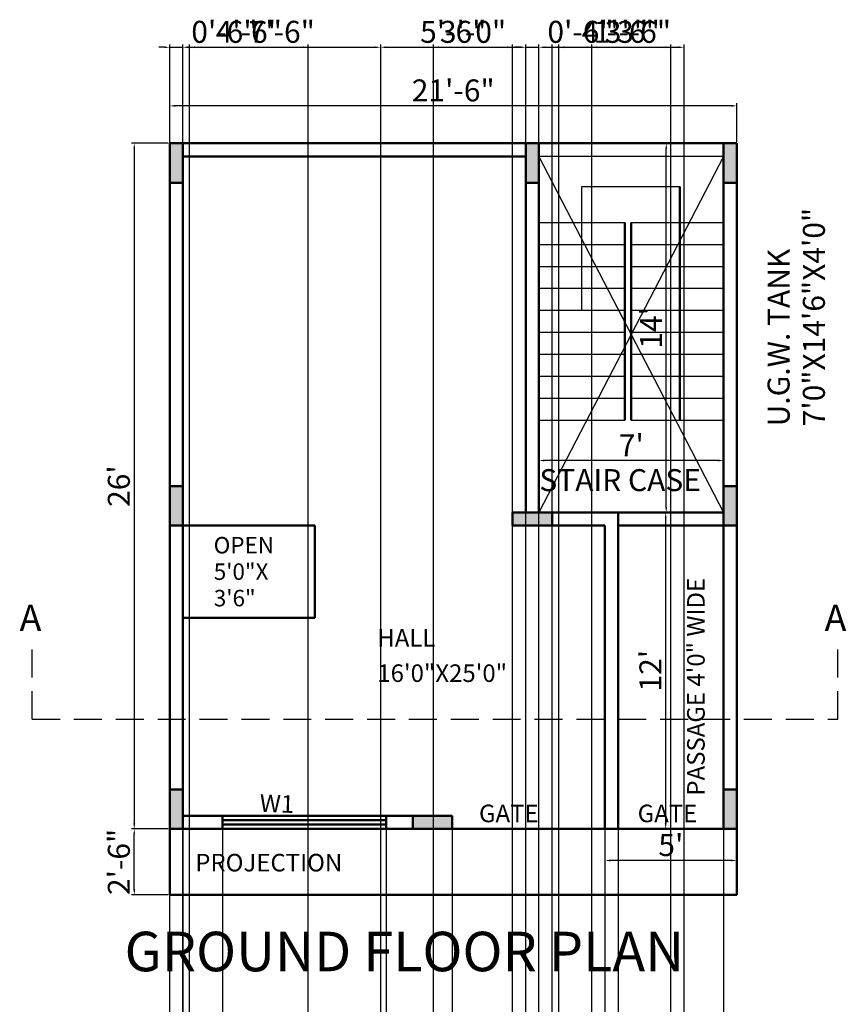
# Model space of a CAD drawing. Units: inches. Extents: x 2368 to 3882, y 1243 to 2139.
# Tile 3 of 6: x 2418 to 2794, y 1691 to 2139. Entities that reach past the tile are written whole.
import ezdxf

# ---------------------------------------------------------------- set-up
doc = ezdxf.new("R2010")
doc.units = ezdxf.units.IN
doc.linetypes.add('DASHED', pattern=[19.05, 12.7, -6.35])
for name, color, linetype, lineweight in [('A-ANNO-DIMS', 2, 'Continuous', 18), ('A-ANNO-SYMB', 1, 'DASHED', 25), ('A-ANNO-TEXT', 7, 'Continuous', 18), ('A-AREA-IDEN', 3, 'Continuous', 18), ('A-FLOR-STRS', 3, 'Continuous', 25), ('A-WALL', 7, 'Continuous', 50), ('A-WALL-PATT', 8, 'Continuous', 13)]:
    doc.layers.add(name, color=color, linetype=linetype, lineweight=lineweight)
doc.styles.get("Standard").update_dxf_attribs({"font": 'arial.ttf'})
doc.dimstyles.new('ISO-25', dxfattribs={"dimtxt": 10, "dimasz": 2.5, "dimexe": 1.25, "dimexo": 0.625, "dimtad": 1, "dimlunit": 3, "dimtxsty": 'Standard', "dimcen": 2.5, "dimadec": 0, "dimazin": 0, "dimtfac": 1, "dimtmove": 0, "dimatfit": 3, "dimfxl": 1, "dimarcsym": 0})

# ---------------------------------------------------------------- blocks, each defined once
blk = doc.blocks.new('*D1')
at = {"layer": 'A-ANNO-DIMS', "color": 0, "lineweight": -2, "transparency": 16777216}
for p, q in [((2486.5, 2083.43), (2486.5, 2101.09)), ((2742, 2099.84), (2489, 2099.84)), ((2744.5, 2083.43), (2744.5, 2101.09))]:
    blk.add_line(p, q, dxfattribs=at)
at = {"layer": 'A-ANNO-DIMS', "color": 0, "transparency": 16777216}
for points in [[(2489, 2100.26), (2489, 2099.43), (2486.5, 2099.84)], [(2742, 2100.26), (2742, 2099.43), (2744.5, 2099.84)]]:
    blk.add_solid(points, dxfattribs=at)
at = {"layer": 'Defpoints', "color": 0, "transparency": 16777216}
for p in [(2486.5, 2099.84), (2486.5, 2082.81), (2744.5, 2082.81)]:
    blk.add_point(p, dxfattribs=at)
at = {"layer": 'A-ANNO-DIMS', "color": 0, "transparency": 16777216, "insert": (2615.5, 2105.57), "char_height": 10, "attachment_point": 5}
blk.add_mtext('21\'-6"', dxfattribs=at)
blk = doc.blocks.new('*D2')
at = {"layer": 'A-ANNO-DIMS', "color": 0, "lineweight": -2, "transparency": 16777216}
for p, q in [((2654.5, 2076.18), (2654.5, 1937.22)), ((2738.5, 2076.18), (2738.5, 1937.22)), ((2736, 1938.47), (2657, 1938.47))]:
    blk.add_line(p, q, dxfattribs=at)
at = {"layer": 'A-ANNO-DIMS', "color": 0, "transparency": 16777216}
for points in [[(2657, 1938.88), (2657, 1938.05), (2654.5, 1938.47)], [(2736, 1938.88), (2736, 1938.05), (2738.5, 1938.47)]]:
    blk.add_solid(points, dxfattribs=at)
at = {"layer": 'Defpoints', "color": 0, "transparency": 16777216}
for p in [(2654.5, 2076.81), (2738.5, 2076.81), (2654.5, 1938.47)]:
    blk.add_point(p, dxfattribs=at)
at = {"layer": 'A-ANNO-DIMS', "color": 0, "transparency": 16777216, "insert": (2696.5, 1944.09), "char_height": 10, "attachment_point": 5}
blk.add_mtext("7'", dxfattribs=at)
blk = doc.blocks.new('*D3')
at = {"layer": 'A-ANNO-DIMS', "color": 0, "lineweight": -2, "transparency": 16777216}
for p, q in [((2649.12, 2082.81), (2713.65, 2082.81)), ((2712.4, 1917.31), (2712.4, 2080.31)), ((2649.12, 1914.81), (2713.65, 1914.81))]:
    blk.add_line(p, q, dxfattribs=at)
at = {"layer": 'A-ANNO-DIMS', "color": 0, "transparency": 16777216}
for points in [[(2711.99, 2080.31), (2712.82, 2080.31), (2712.4, 2082.81)], [(2711.99, 1917.31), (2712.82, 1917.31), (2712.4, 1914.81)]]:
    blk.add_solid(points, dxfattribs=at)
at = {"layer": 'Defpoints', "color": 0, "transparency": 16777216}
for p in [(2648.5, 2082.81), (2712.4, 2082.81), (2648.5, 1914.81)]:
    blk.add_point(p, dxfattribs=at)
at = {"layer": 'A-ANNO-DIMS', "color": 0, "transparency": 16777216, "insert": (2706.76, 1998.81), "char_height": 10, "attachment_point": 5, "rotation": 90}
blk.add_mtext("14'", dxfattribs=at)
blk = doc.blocks.new('*D4')
at = {"layer": 'A-ANNO-DIMS', "color": 0, "lineweight": -2, "transparency": 16777216}
for p, q in [((2485.87, 2082.81), (2469.15, 2082.81)), ((2470.4, 2080.31), (2470.4, 1773.31)), ((2485.87, 1770.81), (2469.15, 1770.81))]:
    blk.add_line(p, q, dxfattribs=at)
at = {"layer": 'A-ANNO-DIMS', "color": 0, "transparency": 16777216}
for points in [[(2469.98, 2080.31), (2470.82, 2080.31), (2470.4, 2082.81)], [(2469.98, 1773.31), (2470.82, 1773.31), (2470.4, 1770.81)]]:
    blk.add_solid(points, dxfattribs=at)
at = {"layer": 'Defpoints', "color": 0, "transparency": 16777216}
for p in [(2486.5, 2082.81), (2470.4, 1770.81), (2486.5, 1770.81)]:
    blk.add_point(p, dxfattribs=at)
at = {"layer": 'A-ANNO-DIMS', "color": 0, "transparency": 16777216, "insert": (2464.67, 1926.81), "char_height": 10, "attachment_point": 5, "rotation": 90}
blk.add_mtext("26'", dxfattribs=at)
blk = doc.blocks.new('*D5')
at = {"layer": 'A-ANNO-DIMS', "color": 0, "lineweight": -2, "transparency": 16777216}
for p, q in [((2485.87, 1770.81), (2469.15, 1770.81)), ((2470.4, 1743.31), (2470.4, 1768.31)), ((2485.87, 1740.81), (2469.15, 1740.81))]:
    blk.add_line(p, q, dxfattribs=at)
at = {"layer": 'A-ANNO-DIMS', "color": 0, "transparency": 16777216}
for points in [[(2469.98, 1768.31), (2470.82, 1768.31), (2470.4, 1770.81)], [(2469.98, 1743.31), (2470.82, 1743.31), (2470.4, 1740.81)]]:
    blk.add_solid(points, dxfattribs=at)
at = {"layer": 'Defpoints', "color": 0, "transparency": 16777216}
for p in [(2470.4, 1770.81), (2486.5, 1770.81), (2486.5, 1740.81)]:
    blk.add_point(p, dxfattribs=at)
at = {"layer": 'A-ANNO-DIMS', "color": 0, "transparency": 16777216, "insert": (2464.67, 1755.81), "char_height": 10, "attachment_point": 5, "rotation": 90}
blk.add_mtext('2\'-6"', dxfattribs=at)
blk = doc.blocks.new('*D6')
at = {"layer": 'A-ANNO-DIMS', "color": 0, "lineweight": -2, "transparency": 16777216}
for p, q in [((2684.5, 1770.18), (2684.5, 1755.19)), ((2744.5, 1770.18), (2744.5, 1755.19)), ((2742, 1756.44), (2687, 1756.44))]:
    blk.add_line(p, q, dxfattribs=at)
at = {"layer": 'A-ANNO-DIMS', "color": 0, "transparency": 16777216}
for points in [[(2687, 1756.85), (2687, 1756.02), (2684.5, 1756.44)], [(2742, 1756.85), (2742, 1756.02), (2744.5, 1756.44)]]:
    blk.add_solid(points, dxfattribs=at)
at = {"layer": 'Defpoints', "color": 0, "transparency": 16777216}
for p in [(2684.5, 1770.81), (2744.5, 1770.81), (2684.5, 1756.44)]:
    blk.add_point(p, dxfattribs=at)
at = {"layer": 'A-ANNO-DIMS', "color": 0, "transparency": 16777216, "insert": (2714.5, 1762.15), "char_height": 10, "attachment_point": 5}
blk.add_mtext("5'", dxfattribs=at)
blk = doc.blocks.new('*D7')
at = {"layer": 'A-ANNO-DIMS', "color": 0, "lineweight": -2, "transparency": 16777216}
for p, q in [((2691.12, 1914.81), (2713.39, 1914.81)), ((2712.14, 1773.31), (2712.14, 1912.31)), ((2691.12, 1770.81), (2713.39, 1770.81))]:
    blk.add_line(p, q, dxfattribs=at)
at = {"layer": 'A-ANNO-DIMS', "color": 0, "transparency": 16777216}
for points in [[(2711.72, 1912.31), (2712.55, 1912.31), (2712.14, 1914.81)], [(2711.72, 1773.31), (2712.55, 1773.31), (2712.14, 1770.81)]]:
    blk.add_solid(points, dxfattribs=at)
at = {"layer": 'Defpoints', "color": 0, "transparency": 16777216}
for p in [(2690.5, 1914.81), (2712.14, 1914.81), (2690.5, 1770.81)]:
    blk.add_point(p, dxfattribs=at)
at = {"layer": 'A-ANNO-DIMS', "color": 0, "transparency": 16777216, "insert": (2706.49, 1842.81), "char_height": 10, "attachment_point": 5, "rotation": 90}
blk.add_mtext("12'", dxfattribs=at)
blk = doc.blocks.new('*D32')
at = {"layer": 'A-ANNO-DIMS', "color": 0, "lineweight": -2, "transparency": 16777216}
for p, q in [((2484, 2126.51), (2481.5, 2126.51)), ((2486.5, 1909.43), (2486.5, 2127.76)), ((2486.5, 2126.51), (2492.5, 2126.51)), ((2492.5, 1909.43), (2492.5, 2127.76)), ((2495, 2126.51), (2525.33, 2126.51))]:
    blk.add_line(p, q, dxfattribs=at)
at = {"layer": 'A-ANNO-DIMS', "color": 0, "transparency": 16777216}
for points in [[(2484, 2126.93), (2484, 2126.09), (2486.5, 2126.51)], [(2495, 2126.93), (2495, 2126.09), (2492.5, 2126.51)]]:
    blk.add_solid(points, dxfattribs=at)
at = {"layer": 'Defpoints', "color": 0, "transparency": 16777216}
for p in [(2492.5, 2126.51), (2486.5, 1908.81), (2492.5, 1908.81)]:
    blk.add_point(p, dxfattribs=at)
at = {"layer": 'A-ANNO-DIMS', "color": 0, "transparency": 16777216, "insert": (2511.41, 2132.24), "char_height": 10, "attachment_point": 5}
blk.add_mtext('0\'-6"', dxfattribs=at)
blk = doc.blocks.new('*D33')
at = {"layer": 'A-ANNO-DIMS', "color": 0, "lineweight": -2, "transparency": 16777216}
for p, q in [((2510.5, 1776.18), (2510.5, 1251.93)), ((2492.5, 1770.18), (2492.5, 1251.93)), ((2495, 1253.18), (2508, 1253.18)), ((2510.5, 1253.18), (2539.89, 1253.18))]:
    blk.add_line(p, q, dxfattribs=at)
at = {"layer": 'A-ANNO-DIMS', "color": 0, "transparency": 16777216}
for points in [[(2495, 1253.6), (2495, 1252.77), (2492.5, 1253.18)], [(2508, 1253.6), (2508, 1252.77), (2510.5, 1253.18)]]:
    blk.add_solid(points, dxfattribs=at)
at = {"layer": 'Defpoints', "color": 0, "transparency": 16777216}
for p in [(2510.5, 1776.81), (2492.5, 1770.81), (2510.5, 1253.18)]:
    blk.add_point(p, dxfattribs=at)
at = {"layer": 'A-ANNO-DIMS', "color": 0, "transparency": 16777216, "insert": (2526.44, 1258.91), "char_height": 10, "attachment_point": 5}
blk.add_mtext('1\'-6"', dxfattribs=at)
blk = doc.blocks.new('*D34')
at = {"layer": 'A-ANNO-DIMS', "color": 0, "lineweight": -2, "transparency": 16777216}
for p, q in [((2510.5, 1776.18), (2510.5, 1251.93)), ((2585.04, 1776.18), (2585.04, 1251.93)), ((2513, 1253.18), (2582.54, 1253.18))]:
    blk.add_line(p, q, dxfattribs=at)
at = {"layer": 'A-ANNO-DIMS', "color": 0, "transparency": 16777216}
for points in [[(2513, 1253.6), (2513, 1252.77), (2510.5, 1253.18)], [(2582.54, 1253.6), (2582.54, 1252.77), (2585.04, 1253.18)]]:
    blk.add_solid(points, dxfattribs=at)
at = {"layer": 'Defpoints', "color": 0, "transparency": 16777216}
for p in [(2510.5, 1776.81), (2585.04, 1776.81), (2585.04, 1253.18)]:
    blk.add_point(p, dxfattribs=at)
at = {"layer": 'A-ANNO-DIMS', "color": 0, "transparency": 16777216, "insert": (2547.77, 1258.98), "char_height": 10, "attachment_point": 5}
blk.add_mtext('6\'-2 1/2"', dxfattribs=at)
blk = doc.blocks.new('*D35')
at = {"layer": 'A-ANNO-DIMS', "color": 0, "lineweight": -2, "transparency": 16777216}
for p, q in [((2585.04, 1776.18), (2585.04, 1251.93)), ((2615.04, 1776.18), (2615.04, 1251.93)), ((2587.54, 1253.18), (2612.54, 1253.18))]:
    blk.add_line(p, q, dxfattribs=at)
at = {"layer": 'A-ANNO-DIMS', "color": 0, "transparency": 16777216}
for points in [[(2587.54, 1253.6), (2587.54, 1252.77), (2585.04, 1253.18)], [(2612.54, 1253.6), (2612.54, 1252.77), (2615.04, 1253.18)]]:
    blk.add_solid(points, dxfattribs=at)
at = {"layer": 'Defpoints', "color": 0, "transparency": 16777216}
for p in [(2585.04, 1776.81), (2615.04, 1776.81), (2615.04, 1253.18)]:
    blk.add_point(p, dxfattribs=at)
at = {"layer": 'A-ANNO-DIMS', "color": 0, "transparency": 16777216, "insert": (2600.04, 1258.91), "char_height": 10, "attachment_point": 5}
blk.add_mtext('2\'-6"', dxfattribs=at)
blk = doc.blocks.new('*D36')
at = {"layer": 'A-ANNO-DIMS', "color": 0, "lineweight": -2, "transparency": 16777216}
for p, q in [((2615.04, 1776.18), (2615.04, 1251.93)), ((2684.5, 1770.18), (2684.5, 1251.93)), ((2617.54, 1253.18), (2682, 1253.18))]:
    blk.add_line(p, q, dxfattribs=at)
at = {"layer": 'A-ANNO-DIMS', "color": 0, "transparency": 16777216}
for points in [[(2617.54, 1253.6), (2617.54, 1252.77), (2615.04, 1253.18)], [(2682, 1253.6), (2682, 1252.77), (2684.5, 1253.18)]]:
    blk.add_solid(points, dxfattribs=at)
at = {"layer": 'Defpoints', "color": 0, "transparency": 16777216}
for p in [(2615.04, 1776.81), (2684.5, 1770.81), (2684.5, 1253.18)]:
    blk.add_point(p, dxfattribs=at)
at = {"layer": 'A-ANNO-DIMS', "color": 0, "transparency": 16777216, "insert": (2649.77, 1258.98), "char_height": 10, "attachment_point": 5}
blk.add_mtext('5\'-9 1/2"', dxfattribs=at)
blk = doc.blocks.new('*D37')
at = {"layer": 'A-ANNO-DIMS', "color": 0, "lineweight": -2, "transparency": 16777216}
for p, q in [((2690.5, 1770.18), (2690.5, 1251.93)), ((2738.5, 1770.18), (2738.5, 1251.93)), ((2693, 1253.18), (2736, 1253.18))]:
    blk.add_line(p, q, dxfattribs=at)
at = {"layer": 'A-ANNO-DIMS', "color": 0, "transparency": 16777216}
for points in [[(2693, 1253.6), (2693, 1252.77), (2690.5, 1253.18)], [(2736, 1253.6), (2736, 1252.77), (2738.5, 1253.18)]]:
    blk.add_solid(points, dxfattribs=at)
at = {"layer": 'Defpoints', "color": 0, "transparency": 16777216}
for p in [(2690.5, 1770.81), (2738.5, 1770.81), (2738.5, 1253.18)]:
    blk.add_point(p, dxfattribs=at)
at = {"layer": 'A-ANNO-DIMS', "color": 0, "transparency": 16777216, "insert": (2714.5, 1258.91), "char_height": 10, "attachment_point": 5}
blk.add_mtext('4\'-0"', dxfattribs=at)
blk = doc.blocks.new('*D39')
at = {"layer": 'A-ANNO-DIMS', "color": 0, "lineweight": -2, "transparency": 16777216}
for p, q in [((2484, 2126.51), (2481.5, 2126.51)), ((2486.5, 1639.51), (2486.5, 2127.76)), ((2486.5, 2126.51), (2492.5, 2126.51)), ((2492.5, 1633.51), (2492.5, 2127.76)), ((2495, 2126.51), (2525.33, 2126.51))]:
    blk.add_line(p, q, dxfattribs=at)
at = {"layer": 'A-ANNO-DIMS', "color": 0, "transparency": 16777216}
for points in [[(2484, 2126.93), (2484, 2126.09), (2486.5, 2126.51)], [(2495, 2126.93), (2495, 2126.09), (2492.5, 2126.51)]]:
    blk.add_solid(points, dxfattribs=at)
at = {"layer": 'Defpoints', "color": 0, "transparency": 16777216}
for p in [(2492.5, 2126.51), (2486.5, 1638.88), (2492.5, 1632.88)]:
    blk.add_point(p, dxfattribs=at)
at = {"layer": 'A-ANNO-DIMS', "color": 0, "transparency": 16777216, "insert": (2511.41, 2132.24), "char_height": 10, "attachment_point": 5}
blk.add_mtext('0\'-6"', dxfattribs=at)
blk = doc.blocks.new('*D50')
at = {"layer": 'A-ANNO-DIMS', "color": 0, "lineweight": -2, "transparency": 16777216}
for p, q in [((2582.5, 1633.51), (2582.5, 2127.76)), ((2585, 2126.51), (2646, 2126.51)), ((2648.5, 1639.51), (2648.5, 2127.76))]:
    blk.add_line(p, q, dxfattribs=at)
at = {"layer": 'A-ANNO-DIMS', "color": 0, "transparency": 16777216}
for points in [[(2585, 2126.93), (2585, 2126.09), (2582.5, 2126.51)], [(2646, 2126.93), (2646, 2126.09), (2648.5, 2126.51)]]:
    blk.add_solid(points, dxfattribs=at)
at = {"layer": 'Defpoints', "color": 0, "transparency": 16777216}
for p in [(2648.5, 2126.51), (2648.5, 1638.88), (2582.5, 1632.88)]:
    blk.add_point(p, dxfattribs=at)
at = {"layer": 'A-ANNO-DIMS', "color": 0, "transparency": 16777216, "insert": (2615.5, 2132.24), "char_height": 10, "attachment_point": 5}
blk.add_mtext('5\'-6"', dxfattribs=at)
blk = doc.blocks.new('*D51')
at = {"layer": 'A-ANNO-DIMS', "color": 0, "lineweight": -2, "transparency": 16777216}
for p, q in [((2646, 2126.51), (2643.5, 2126.51)), ((2648.5, 1639.51), (2648.5, 2127.76)), ((2648.5, 2126.51), (2654.5, 2126.51)), ((2654.5, 1639.51), (2654.5, 2127.76)), ((2657, 2126.51), (2687.33, 2126.51))]:
    blk.add_line(p, q, dxfattribs=at)
at = {"layer": 'A-ANNO-DIMS', "color": 0, "transparency": 16777216}
for points in [[(2646, 2126.93), (2646, 2126.09), (2648.5, 2126.51)], [(2657, 2126.93), (2657, 2126.09), (2654.5, 2126.51)]]:
    blk.add_solid(points, dxfattribs=at)
at = {"layer": 'Defpoints', "color": 0, "transparency": 16777216}
for p in [(2654.5, 2126.51), (2648.5, 1638.88), (2654.5, 1638.88)]:
    blk.add_point(p, dxfattribs=at)
at = {"layer": 'A-ANNO-DIMS', "color": 0, "transparency": 16777216, "insert": (2673.41, 2132.24), "char_height": 10, "attachment_point": 5}
blk.add_mtext('0\'-6"', dxfattribs=at)
blk = doc.blocks.new('*D52')
at = {"layer": 'A-ANNO-DIMS', "color": 0, "lineweight": -2, "transparency": 16777216}
for p, q in [((2492.5, 1633.51), (2492.5, 2127.76)), ((2495, 2126.51), (2580, 2126.51)), ((2582.5, 1633.51), (2582.5, 2127.76))]:
    blk.add_line(p, q, dxfattribs=at)
at = {"layer": 'A-ANNO-DIMS', "color": 0, "transparency": 16777216}
for points in [[(2495, 2126.93), (2495, 2126.09), (2492.5, 2126.51)], [(2580, 2126.93), (2580, 2126.09), (2582.5, 2126.51)]]:
    blk.add_solid(points, dxfattribs=at)
at = {"layer": 'Defpoints', "color": 0, "transparency": 16777216}
for p in [(2582.5, 2126.51), (2492.5, 1632.88), (2582.5, 1632.88)]:
    blk.add_point(p, dxfattribs=at)
at = {"layer": 'A-ANNO-DIMS', "color": 0, "transparency": 16777216, "insert": (2537.5, 2132.24), "char_height": 10, "attachment_point": 5}
blk.add_mtext('7\'-6"', dxfattribs=at)
blk = doc.blocks.new('*D53')
at = {"layer": 'A-ANNO-DIMS', "color": 0, "lineweight": -2, "transparency": 16777216}
for p, q in [((2663.5, 1357.51), (2663.5, 2127.76)), ((2666, 2126.51), (2712, 2126.51)), ((2714.5, 1357.51), (2714.5, 2127.76))]:
    blk.add_line(p, q, dxfattribs=at)
at = {"layer": 'A-ANNO-DIMS', "color": 0, "transparency": 16777216}
for points in [[(2666, 2126.93), (2666, 2126.09), (2663.5, 2126.51)], [(2712, 2126.93), (2712, 2126.09), (2714.5, 2126.51)]]:
    blk.add_solid(points, dxfattribs=at)
at = {"layer": 'Defpoints', "color": 0, "transparency": 16777216}
for p in [(2714.5, 2126.51), (2663.5, 1356.88), (2714.5, 1356.88)]:
    blk.add_point(p, dxfattribs=at)
at = {"layer": 'A-ANNO-DIMS', "color": 0, "transparency": 16777216, "insert": (2689, 2132.24), "char_height": 10, "attachment_point": 5}
blk.add_mtext('4\'-3"', dxfattribs=at)
blk = doc.blocks.new('*D58')
at = {"layer": 'A-ANNO-DIMS', "color": 0, "lineweight": -2, "transparency": 16777216}
for p, q in [((2495.5, 1471.51), (2495.5, 2127.76)), ((2498, 2126.51), (2547, 2126.51)), ((2549.5, 1471.51), (2549.5, 2127.76))]:
    blk.add_line(p, q, dxfattribs=at)
at = {"layer": 'A-ANNO-DIMS', "color": 0, "transparency": 16777216}
for points in [[(2498, 2126.93), (2498, 2126.09), (2495.5, 2126.51)], [(2547, 2126.93), (2547, 2126.09), (2549.5, 2126.51)]]:
    blk.add_solid(points, dxfattribs=at)
at = {"layer": 'Defpoints', "color": 0, "transparency": 16777216}
for p in [(2549.5, 2126.51), (2495.5, 1470.88), (2549.5, 1470.88)]:
    blk.add_point(p, dxfattribs=at)
at = {"layer": 'A-ANNO-DIMS', "color": 0, "transparency": 16777216, "insert": (2522.5, 2132.24), "char_height": 10, "attachment_point": 5}
blk.add_mtext('4\'-6"', dxfattribs=at)
blk = doc.blocks.new('*D59')
at = {"layer": 'A-ANNO-DIMS', "color": 0, "lineweight": -2, "transparency": 16777216}
for p, q in [((2606.5, 1465.51), (2606.5, 2127.76)), ((2609, 2126.51), (2640, 2126.51)), ((2642.5, 1471.51), (2642.5, 2127.76))]:
    blk.add_line(p, q, dxfattribs=at)
at = {"layer": 'A-ANNO-DIMS', "color": 0, "transparency": 16777216}
for points in [[(2609, 2126.93), (2609, 2126.09), (2606.5, 2126.51)], [(2640, 2126.93), (2640, 2126.09), (2642.5, 2126.51)]]:
    blk.add_solid(points, dxfattribs=at)
at = {"layer": 'Defpoints', "color": 0, "transparency": 16777216}
for p in [(2642.5, 2126.51), (2642.5, 1470.88), (2606.5, 1464.88)]:
    blk.add_point(p, dxfattribs=at)
at = {"layer": 'A-ANNO-DIMS', "color": 0, "transparency": 16777216, "insert": (2624.5, 2132.24), "char_height": 10, "attachment_point": 5}
blk.add_mtext('3\'-0"', dxfattribs=at)
blk = doc.blocks.new('*D60')
at = {"layer": 'A-ANNO-DIMS', "color": 0, "lineweight": -2, "transparency": 16777216}
for p, q in [((2660.5, 1471.51), (2660.5, 2127.76)), ((2663, 2126.51), (2676, 2126.51)), ((2678.5, 1471.51), (2678.5, 2127.76)), ((2678.5, 2126.51), (2707.89, 2126.51))]:
    blk.add_line(p, q, dxfattribs=at)
at = {"layer": 'A-ANNO-DIMS', "color": 0, "transparency": 16777216}
for points in [[(2663, 2126.93), (2663, 2126.09), (2660.5, 2126.51)], [(2676, 2126.93), (2676, 2126.09), (2678.5, 2126.51)]]:
    blk.add_solid(points, dxfattribs=at)
at = {"layer": 'Defpoints', "color": 0, "transparency": 16777216}
for p in [(2678.5, 2126.51), (2660.5, 1470.88), (2678.5, 1470.88)]:
    blk.add_point(p, dxfattribs=at)
at = {"layer": 'A-ANNO-DIMS', "color": 0, "transparency": 16777216, "insert": (2694.44, 2132.24), "char_height": 10, "attachment_point": 5}
blk.add_mtext('1\'-6"', dxfattribs=at)
blk = doc.blocks.new('*D61')
at = {"layer": 'A-ANNO-DIMS', "color": 0, "lineweight": -2, "transparency": 16777216}
for p, q in [((2678.5, 1471.51), (2678.5, 2127.76)), ((2681, 2126.51), (2718, 2126.51)), ((2720.5, 1471.51), (2720.5, 2127.76))]:
    blk.add_line(p, q, dxfattribs=at)
at = {"layer": 'A-ANNO-DIMS', "color": 0, "transparency": 16777216}
for points in [[(2681, 2126.93), (2681, 2126.09), (2678.5, 2126.51)], [(2718, 2126.93), (2718, 2126.09), (2720.5, 2126.51)]]:
    blk.add_solid(points, dxfattribs=at)
at = {"layer": 'Defpoints', "color": 0, "transparency": 16777216}
for p in [(2720.5, 2126.51), (2678.5, 1470.88), (2720.5, 1470.88)]:
    blk.add_point(p, dxfattribs=at)
at = {"layer": 'A-ANNO-DIMS', "color": 0, "transparency": 16777216, "insert": (2699.5, 2132.24), "char_height": 10, "attachment_point": 5}
blk.add_mtext('3\'-6"', dxfattribs=at)

msp = doc.modelspace()

# ---------------------------------------------------------------- hatches: boundary and pattern name
at = {"layer": 'A-WALL-PATT'}
h = msp.add_hatch(color=256, dxfattribs=at)
h.dxf.hatch_style = 1
h.paths.add_polyline_path([(2492.497, 1344.883), (2486.497, 1344.883), (2486.497, 1326.883), (2492.497, 1326.883)])
h.paths.add_polyline_path([(2618.497, 1332.883), (2600.497, 1332.883), (2600.497, 1326.883), (2618.497, 1326.883)])
h.paths.add_polyline_path([(2744.497, 1344.883), (2738.497, 1344.883), (2738.497, 1326.883), (2744.497, 1326.883)])
h.paths.add_polyline_path([(2744.497, 1482.883), (2738.497, 1482.883), (2738.497, 1464.883), (2744.497, 1464.883)])
h.paths.add_polyline_path([(2660.497, 1470.883), (2642.497, 1470.883), (2642.497, 1464.883), (2660.497, 1464.883)])
h.paths.add_polyline_path([(2492.497, 1482.883), (2486.497, 1482.883), (2486.497, 1464.883), (2492.497, 1464.883)])
h.paths.add_polyline_path([(2492.497, 1638.883), (2486.497, 1638.883), (2486.497, 1620.883), (2492.497, 1620.883)])
h.paths.add_polyline_path([(2654.497, 1638.883), (2648.497, 1638.883), (2648.497, 1620.883), (2654.497, 1620.883)])
h.paths.add_polyline_path([(2744.497, 1638.883), (2738.497, 1638.883), (2738.497, 1620.883), (2744.497, 1620.883)])
h.paths.add_polyline_path([(2744.497, 1788.809), (2738.497, 1788.809), (2738.497, 1770.809), (2744.497, 1770.809)])
h.paths.add_polyline_path([(2615.041, 1776.809), (2597.041, 1776.809), (2597.041, 1770.809), (2615.041, 1770.809)])
h.paths.add_polyline_path([(2492.497, 1788.809), (2486.497, 1788.809), (2486.497, 1770.809), (2492.497, 1770.809)])
h.paths.add_polyline_path([(2492.497, 1926.809), (2486.497, 1926.809), (2486.497, 1908.809), (2492.497, 1908.809)])
h.paths.add_polyline_path([(2660.497, 1914.809), (2642.497, 1914.809), (2642.497, 1908.809), (2660.497, 1908.809)])
h.paths.add_polyline_path([(2744.497, 1926.809), (2738.497, 1926.809), (2738.497, 1908.809), (2744.497, 1908.809)])
h.paths.add_polyline_path([(2744.497, 2082.809), (2738.497, 2082.809), (2738.497, 2064.809), (2744.497, 2064.809)])
h.paths.add_polyline_path([(2654.497, 2082.809), (2648.497, 2082.809), (2648.497, 2064.809), (2654.497, 2064.809)])
h.paths.add_polyline_path([(2492.497, 2082.809), (2486.497, 2082.809), (2486.497, 2064.809), (2492.497, 2064.809)])

# ---------------------------------------------------------------- linework, layer by layer
at = {"layer": 'A-ANNO-SYMB'}
for p, q in [((2423.91, 1820.722), (2423.91, 1857.529)), ((2790.406, 1820.722), (2790.406, 1857.529)), ((2423.91, 1820.722), (2790.406, 1820.722))]:
    msp.add_line(p, q, dxfattribs=at)
at = {"layer": 'A-FLOR-STRS'}
for p, q in [((2738.497, 2076.809), (2654.497, 2076.809)), ((2738.497, 2076.809), (2654.497, 1914.809)), ((2654.497, 2076.809), (2738.497, 1914.809)), ((2673.997, 2006.809), (2673.997, 2063.189)), ((2673.997, 2063.189), (2718.522, 2063.189)), ((2654.497, 2046.809), (2693.497, 2046.809)), ((2696.497, 2046.809), (2738.497, 2046.809)), ((2654.497, 2036.809), (2693.497, 2036.809)), ((2696.497, 2036.809), (2738.497, 2036.809)), ((2654.497, 2026.809), (2693.497, 2026.809)), ((2696.497, 2026.809), (2738.497, 2026.809)), ((2654.497, 2016.809), (2693.497, 2016.809)), ((2696.497, 2016.809), (2738.497, 2016.809)), ((2654.497, 2006.809), (2693.497, 2006.809)), ((2696.497, 2006.809), (2738.497, 2006.809)), ((2654.497, 1996.809), (2693.497, 1996.809)), ((2696.497, 1996.809), (2738.497, 1996.809)), ((2654.497, 1986.809), (2693.497, 1986.809)), ((2696.497, 1986.809), (2738.497, 1986.809)), ((2654.497, 1976.809), (2693.497, 1976.809)), ((2696.497, 1976.809), (2738.497, 1976.809)), ((2654.497, 1966.809), (2693.497, 1966.809)), ((2696.497, 1966.809), (2738.497, 1966.809)), ((2654.497, 1956.809), (2693.497, 1956.809)), ((2696.497, 1956.809), (2738.497, 1956.809))]:
    msp.add_line(p, q, dxfattribs=at)
at = {"layer": 'A-WALL'}
for p, q in [((2744.497, 2082.809), (2486.497, 2082.809)), ((2486.497, 2082.809), (2486.497, 1770.809)), ((2492.497, 2082.809), (2492.497, 1770.809)), ((2648.497, 1914.809), (2648.497, 2082.809)), ((2654.497, 1914.809), (2654.497, 2082.809)), ((2738.497, 1770.809), (2738.497, 2082.809)), ((2744.497, 1740.809), (2744.497, 2082.809)), ((2648.497, 2076.809), (2492.497, 2076.809)), ((2492.497, 2064.809), (2486.497, 2064.809)), ((2654.497, 2064.809), (2648.497, 2064.809)), ((2718.522, 2063.189), (2718.522, 1956.809)), ((2744.497, 2064.809), (2738.497, 2064.809)), ((2693.497, 1956.809), (2693.497, 2046.809)), ((2696.497, 1956.809), (2696.497, 2046.809)), ((2492.497, 1926.809), (2486.497, 1926.809)), ((2744.497, 1926.809), (2738.497, 1926.809)), ((2642.497, 1914.809), (2738.497, 1914.809)), ((2642.497, 1914.809), (2642.497, 1908.809)), ((2660.497, 1914.809), (2660.497, 1908.809)), ((2690.497, 1770.809), (2690.497, 1914.809)), ((2492.497, 1908.809), (2486.497, 1908.809)), ((2492.497, 1908.809), (2552.497, 1908.809)), ((2552.497, 1908.809), (2552.497, 1866.809)), ((2642.497, 1908.809), (2684.497, 1908.809)), ((2684.497, 1770.809), (2684.497, 1908.809)), ((2690.497, 1908.809), (2738.497, 1908.809)), ((2744.497, 1908.809), (2738.497, 1908.809)), ((2492.497, 1866.809), (2552.497, 1866.809)), ((2492.497, 1788.809), (2486.497, 1788.809)), ((2744.497, 1788.809), (2738.497, 1788.809)), ((2492.497, 1776.809), (2615.041, 1776.809)), ((2510.497, 1776.809), (2510.497, 1770.809)), ((2510.497, 1774.809), (2585.041, 1774.809)), ((2585.041, 1776.809), (2585.041, 1770.809)), ((2597.041, 1776.809), (2597.041, 1770.809)), ((2615.041, 1776.809), (2615.041, 1770.809)), ((2486.497, 1770.809), (2684.497, 1770.809)), ((2486.497, 1740.809), (2486.497, 1770.809)), ((2510.497, 1772.809), (2585.041, 1772.809)), ((2744.497, 1770.809), (2684.497, 1770.809)), ((2486.497, 1740.809), (2744.497, 1740.809))]:
    msp.add_line(p, q, dxfattribs=at)

# ---------------------------------------------------------------- texts
at = {"layer": 'A-ANNO-SYMB'}
for p in [(2418.21, 1860.827), (2784.415, 1860.827)]:
    msp.add_text('A', height=12, dxfattribs=at).set_placement(p)
at = {"layer": 'A-ANNO-TEXT'}
msp.add_text('W1', height=8, rotation=358.08049, dxfattribs=at).set_placement((2527.353, 1778.584))
for s, height, p in [('GATE', 8, (2627.213, 1773.854)), ('GATE', 8, (2699.394, 1773.854)), ('GROUND FLOOR PLAN', 18, (2465.996, 1706.018))]:
    msp.add_text(s, height=height, dxfattribs=at).set_placement(p)
at = {"layer": 'A-AREA-IDEN'}
for s, height, rotation, p in [('7\'0"X14\'6"X4\'0"', 10, 90, (2784.562, 1954.022)), ('U.G.W. TANK', 10, 90, (2768.498, 1954.022)), ('OPEN', 7.4943, 0.16667, (2506.521, 1896.152)), ('5\'0"X', 7.4943, 0.16667, (2506.556, 1884.113)), ('PASSAGE 4\'0" WIDE', 8, 90, (2729.887, 1785.973)), ('3\'6"', 7.4943, 0.16667, (2506.591, 1872.074))]:
    msp.add_text(s, height=height, rotation=rotation, dxfattribs=at).set_placement(p)
for s, height, p in [('STAIR CASE', 10, (2654.672, 1924.524)), ('HALL', 8, (2580.964, 1853.737)), ('16\'0"X25\'0"', 8, (2580.964, 1837.673)), ('PROJECTION', 8, (2498.128, 1751.457))]:
    msp.add_text(s, height=height, dxfattribs=at).set_placement(p)

# ---------------------------------------------------------------- dimensions: what is measured, and where the dimension line sits
at = {"layer": 'A-ANNO-DIMS'}
for base, p1, p2, override, picture, middle in [((2492.497, 2126.509), (2486.497, 1908.809), (2492.497, 1908.809), {"dimdec": 1, "dimlfac": 1, "dimrnd": 0, "dimzin": 1, "dimdsep": 46, "dimlunit": 4, "dimfrac": 2}, '*D32', (2511.414, 2132.24)), ((2492.497, 2126.509), (2486.497, 1638.883), (2492.497, 1632.883), {"dimdec": 1, "dimlfac": 1, "dimrnd": 0, "dimzin": 1, "dimdsep": 46, "dimlunit": 4, "dimfrac": 2}, '*D39', (2511.414, 2132.24)), ((2582.497, 2126.509), (2492.497, 1632.883), (2582.497, 1632.883), {"dimdec": 1, "dimlfac": 1, "dimrnd": 0, "dimzin": 1, "dimdsep": 46, "dimlunit": 4, "dimfrac": 2}, '*D52', (2537.497, 2132.24)), ((2549.497, 2126.509), (2495.497, 1470.883), (2549.497, 1470.883), {"dimdec": 1, "dimlfac": 1, "dimrnd": 0, "dimzin": 1, "dimdsep": 46, "dimlunit": 4, "dimfrac": 2}, '*D58', (2522.497, 2132.24)), ((2648.497, 2126.509), (2582.497, 1632.883), (2648.497, 1638.883), {"dimdec": 1, "dimlfac": 1, "dimrnd": 0, "dimzin": 1, "dimdsep": 46, "dimlunit": 4, "dimfrac": 2}, '*D50', (2615.497, 2132.24)), ((2642.497, 2126.509), (2606.497, 1464.883), (2642.497, 1470.883), {"dimdec": 1, "dimlfac": 1, "dimrnd": 0, "dimzin": 1, "dimdsep": 46, "dimlunit": 4, "dimfrac": 2}, '*D59', (2624.497, 2132.243)), ((2654.497, 2126.509), (2648.497, 1638.883), (2654.497, 1638.883), {"dimdec": 1, "dimlfac": 1, "dimrnd": 0, "dimzin": 1, "dimdsep": 46, "dimlunit": 4, "dimfrac": 2}, '*D51', (2673.414, 2132.24)), ((2678.497, 2126.509), (2660.497, 1470.883), (2678.497, 1470.883), {"dimdec": 1, "dimlfac": 1, "dimrnd": 0, "dimzin": 1, "dimdsep": 46, "dimlunit": 4, "dimfrac": 2}, '*D60', (2694.443, 2132.24)), ((2714.497, 2126.509), (2663.497, 1356.883), (2714.497, 1356.883), {"dimdec": 1, "dimlfac": 1, "dimrnd": 0, "dimzin": 1, "dimdsep": 46, "dimlunit": 4, "dimfrac": 2}, '*D53', (2688.997, 2132.243)), ((2720.497, 2126.509), (2678.497, 1470.883), (2720.497, 1470.883), {"dimdec": 1, "dimlfac": 1, "dimrnd": 0, "dimzin": 1, "dimdsep": 46, "dimlunit": 4, "dimfrac": 2}, '*D61', (2699.497, 2132.243)), ((2486.497, 2099.844), (2744.497, 2082.809), (2486.497, 2082.809), {"dimclrd": 0, "dimclre": 0, "dimclrt": 0}, '*D1', (2615.497, 2105.575)), ((2654.497, 1938.465), (2738.497, 2076.809), (2654.497, 2076.809), {"dimclrd": 0, "dimclre": 0, "dimclrt": 0}, '*D2', (2696.497, 1944.09)), ((2510.497, 1253.183), (2492.497, 1770.809), (2510.497, 1776.809), {"dimdec": 1, "dimlfac": 1, "dimrnd": 0, "dimzin": 1, "dimdsep": 46, "dimlunit": 4, "dimfrac": 2}, '*D33', (2526.443, 1258.914)), ((2585.041, 1253.183), (2510.497, 1776.809), (2585.041, 1776.809), {"dimdec": 1, "dimlfac": 1, "dimrnd": 0, "dimzin": 1, "dimdsep": 46, "dimlunit": 4, "dimfrac": 2}, '*D34', (2547.769, 1258.979)), ((2615.041, 1253.183), (2585.041, 1776.809), (2615.041, 1776.809), {"dimdec": 1, "dimlfac": 1, "dimrnd": 0, "dimzin": 1, "dimdsep": 46, "dimlunit": 4, "dimfrac": 2}, '*D35', (2600.041, 1258.914)), ((2684.497, 1253.183), (2615.041, 1776.809), (2684.497, 1770.809), {"dimdec": 1, "dimlfac": 1, "dimrnd": 0, "dimzin": 1, "dimdsep": 46, "dimlunit": 4, "dimfrac": 2}, '*D36', (2649.769, 1258.979)), ((2684.497, 1756.438), (2744.497, 1770.809), (2684.497, 1770.809), {"dimclrd": 0, "dimclre": 0, "dimclrt": 0}, '*D6', (2714.497, 1762.148)), ((2738.497, 1253.183), (2690.497, 1770.809), (2738.497, 1770.809), {"dimdec": 1, "dimlfac": 1, "dimrnd": 0, "dimzin": 1, "dimdsep": 46, "dimlunit": 4, "dimfrac": 2}, '*D37', (2714.497, 1258.914))]:
    dim = msp.add_linear_dim(base=base, p1=p1, p2=p2, dimstyle='ISO-25', override=override, dxfattribs=at)
    dim.commit()
    dim.dimension.update_dxf_attribs({"geometry": picture, "text_midpoint": middle})
for base, p1, p2, picture, middle in [((2470.399, 1770.809), (2486.497, 2082.809), (2486.497, 1770.809), '*D4', (2464.668, 1926.809)), ((2712.404, 2082.809), (2648.497, 1914.809), (2648.497, 2082.809), '*D3', (2706.758, 1998.809)), ((2712.136, 1914.809), (2690.497, 1770.809), (2690.497, 1914.809), '*D7', (2706.49, 1842.809)), ((2470.4, 1770.809), (2486.497, 1740.809), (2486.497, 1770.809), '*D5', (2464.669, 1755.809))]:
    dim = msp.add_linear_dim(base=base, p1=p1, p2=p2, angle=90, dimstyle='ISO-25', override={"dimclrd": 0, "dimclre": 0, "dimclrt": 0}, dxfattribs=at)
    dim.commit()
    dim.dimension.update_dxf_attribs({"geometry": picture, "text_midpoint": middle})

doc.saveas('drawing.dxf')
